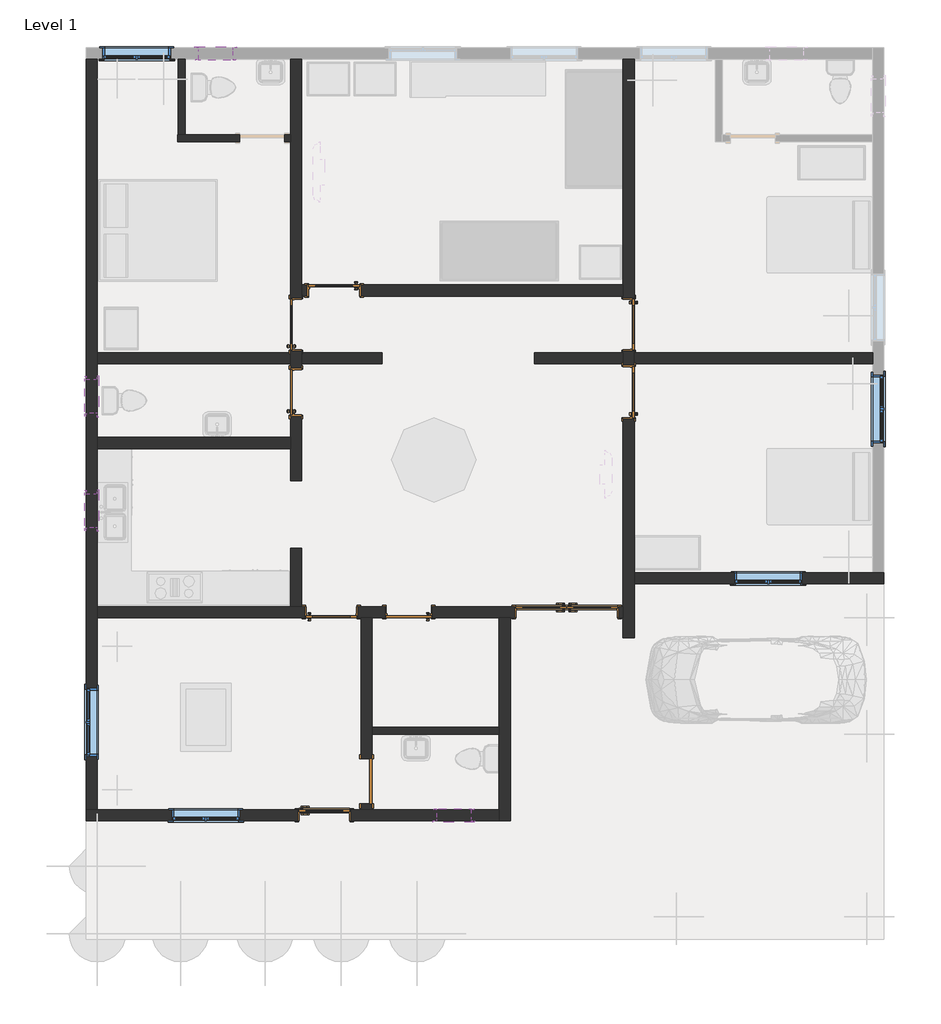
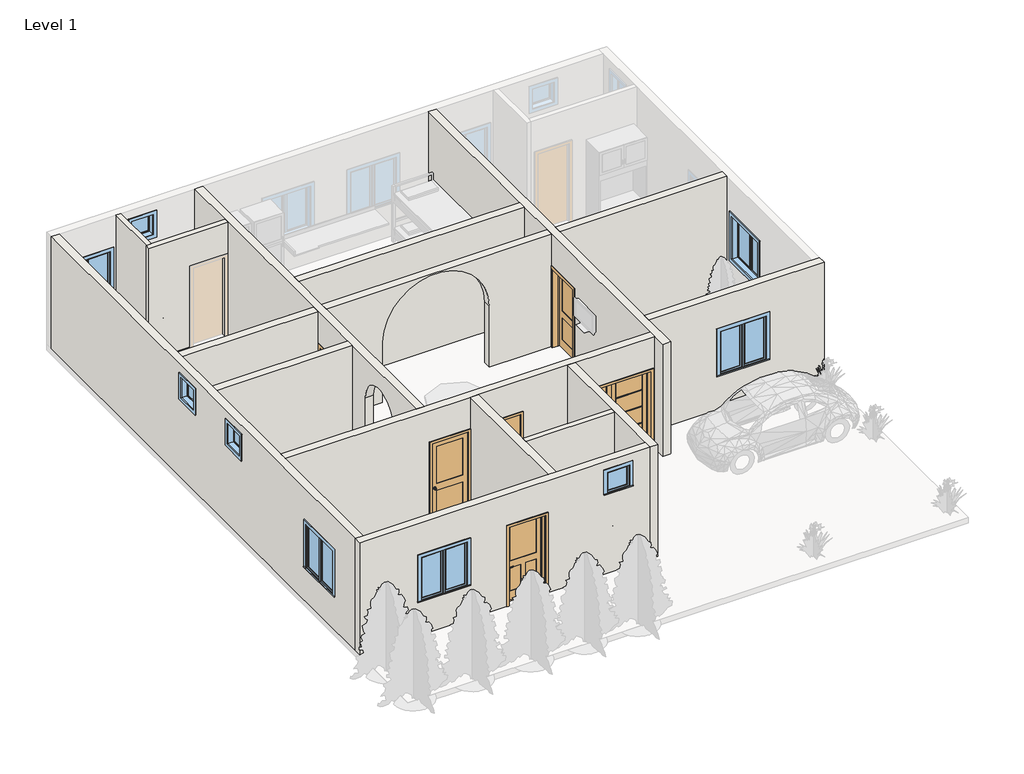
# One storey, part 1 of 2: 14 walls, 10 doors, 9 windows.
"""IFC4 building model written with IfcOpenShell, lengths in millimetres."""

from ifc_helpers import new_model, si_unit, point, frame, frame_2d, origin, origin_with_axes, place, context, project, spatial, polyline, circle_curve, trimmed, segment, composite_curve, outline, extrude, faceted_brep, transform, mapped, element, save
from ifc_brep_helpers import plane_surface, revolved_surface, advanced_brep
from components import door_e879f077, door_06d7e188, door_6f959a6d, door_387d6dd4, door_e4576485, door_70ddef25, window_0862ab64, window_e41d21a6

model = new_model("IFC4")

# Units and contexts
model_context = context("Model", 3, world=origin())
ifc_project = project(units=[si_unit("LENGTHUNIT", "METRE", prefix="MILLI")], contexts=[model_context])

# Site, building, storey
site = spatial("IfcSite", under=ifc_project)
building = spatial("IfcBuilding", under=site)
storey = spatial("IfcBuildingStorey", under=building, Name="Level 1", Elevation=0.0)

# Doors
placement = place(None, origin())
door_shape = door_e879f077(model_context)
element("IfcDoor", 1, ObjectType="36\" x 84\"", at=placement, inside=storey, context=model_context, shape_type="MappedRepresentation", body=[
    mapped(door_shape, transform((1274.4768082, -2194.7262669, 0.0), x_axis=(-1.0, 0.0, 0.0), y_axis=(0.0, -1.0, 0.0), z_axis=(0.0, 0.0, 1.0))),
])
door_2_shape = door_06d7e188(model_context)
element("IfcDoor", 2, ObjectType="Door-Exterior-Double-Full Glass-Wood_Clad : 72\" x 84\"", at=placement, inside=storey, context=model_context, shape_type="MappedRepresentation", body=[
    mapped(door_2_shape, transform((5643.2768082, 1462.8737331, 0.0), x_axis=(1.0, 0.0, 0.0), y_axis=(0.0, 1.0, 0.0), z_axis=(0.0, 0.0, 1.0))),
])
door_3_shape = door_6f959a6d(model_context)
element("IfcDoor", 3, ObjectType="Door-Interior-Single-2_Panel-Wood : 36\" x 84\"", at=placement, inside=storey, context=model_context, shape_type="MappedRepresentation", body=[
    mapped(door_3_shape, transform((6764.0518082, 6641.2987331, 0.0), x_axis=(0.0, -1.0, 0.0), y_axis=(1.0, 0.0, 0.0), z_axis=(0.0, 0.0, 1.0))),
])
element("IfcDoor", 4, ObjectType="Door-Interior-Single-2_Panel-Wood : 36\" x 84\"", at=placement, inside=storey, context=model_context, shape_type="MappedRepresentation", body=[
    mapped(door_3_shape, transform((763.3018082, 6641.2987331, 0.0), x_axis=(0.0, 1.0, 0.0), y_axis=(-1.0, 0.0, 0.0), z_axis=(0.0, 0.0, 1.0))),
])
door_4_shape = door_387d6dd4(model_context)
element("IfcDoor", 5, ObjectType="Door-Interior-Single-2_Panel-Wood : 36\" x 84\"", at=placement, inside=storey, context=model_context, shape_type="MappedRepresentation", body=[
    mapped(door_4_shape, transform((1452.2768082, 7254.0737331, 0.0), x_axis=(-1.0, 0.0, 0.0), y_axis=(0.0, -1.0, 0.0), z_axis=(0.0, 0.0, 1.0))),
])
element("IfcDoor", 6, ObjectType="Door-Interior-Single-2_Panel-Wood : 36\" x 84\"", at=placement, inside=storey, context=model_context, shape_type="MappedRepresentation", body=[
    mapped(door_4_shape, transform((6764.0518082, 5422.0987331, 0.0), x_axis=(0.0, 1.0, 0.0), y_axis=(-1.0, 0.0, 0.0), z_axis=(0.0, 0.0, 1.0))),
])
element("IfcDoor", 7, ObjectType="Door-Interior-Single-2_Panel-Wood : 36\" x 84\"", at=placement, inside=storey, context=model_context, shape_type="MappedRepresentation", body=[
    mapped(door_4_shape, transform((1401.4768082, 1456.5237331, 0.0), x_axis=(1.0, 0.0, 0.0), y_axis=(0.0, 1.0, 0.0), z_axis=(0.0, 0.0, 1.0))),
])
door_5_shape = door_e4576485(model_context)
element("IfcDoor", 8, ObjectType="Door-Interior-Single-Flush_Panel-Wood : 32\" x 84\"", at=placement, inside=storey, context=model_context, shape_type="MappedRepresentation", body=[
    mapped(door_5_shape, transform((763.3018082, 5422.0987331, 0.0), x_axis=(0.0, 1.0, 0.0), y_axis=(-1.0, 0.0, 0.0), z_axis=(0.0, 0.0, 1.0))),
])
element("IfcDoor", 9, ObjectType="Door-Interior-Single-Flush_Panel-Wood : 32\" x 84\"", at=placement, inside=storey, context=model_context, shape_type="MappedRepresentation", body=[
    mapped(door_5_shape, transform((2798.4768082, 1456.5237331, 0.0), x_axis=(-1.0, 0.0, 0.0), y_axis=(0.0, -1.0, 0.0), z_axis=(0.0, 0.0, 1.0))),
])
door_6_shape = door_70ddef25(model_context)
element("IfcDoor", 10, ObjectType="Door-Single-Panel : 32\" x 84\"", at=placement, inside=storey, context=model_context, shape_type="MappedRepresentation", body=[
    mapped(door_6_shape, transform((2036.4768082, -1588.3012669, 0.0), x_axis=(0.0, -1.0, 0.0), y_axis=(1.0, 0.0, 0.0), z_axis=(0.0, 0.0, 1.0))),
])

# Walls
element("IfcWall", 11, ObjectType="Generic - 5\"", at=placement, inside=storey, context=model_context, shape_type="Brep", body=[
    faceted_brep([(563.2768082, 9930.5987331, 2133.6), (563.2768082, 9930.5987331, 0.0), (664.8768082, 9930.5987331, 0.0), (664.8768082, 9930.5987331, 3048.0), (-1367.1231918, 9930.5987331, 3048.0), (-1367.1231918, 9930.5987331, 0.0), (-249.5231918, 9930.5987331, 0.0), (-249.5231918, 9930.5987331, 2133.6), (664.8768082, 10057.5987331, 0.0), (563.2768082, 10057.5987331, 0.0), (563.2768082, 10057.5987331, 2133.6), (-249.5231918, 10057.5987331, 2133.6), (-249.5231918, 10057.5987331, 0.0), (-1227.4231918, 10057.5987331, 0.0), (-1354.4231918, 10057.5987331, 0.0), (-1367.1231918, 10057.5987331, 0.0), (-1367.1231918, 10057.5987331, 3048.0), (-1354.4231918, 10057.5987331, 3048.0), (-1227.4231918, 10057.5987331, 3048.0), (664.8768082, 10057.5987331, 3048.0)], [[[0, 1, 2, 3, 4, 5, 6, 7]], [[8, 9, 10, 11, 12, 13, 14, 15, 16, 17, 18, 19]], [[6, 5, 15, 14, 13, 12]], [[2, 1, 9, 8]], [[4, 3, 19, 18, 17, 16]], [[5, 4, 16, 15]], [[3, 2, 8, 19]], [[10, 9, 1, 0]], [[11, 10, 0, 7]], [[12, 11, 7, 6]]]),
])
element("IfcWall", 12, ObjectType="Generic - 5\"", at=placement, inside=storey, context=model_context, shape_type="SweptSolid", body=[
    extrude(outline(polyline([(-1227.4231918, 11416.4987331), (-1227.4231918, 10057.5987331), (-1354.4231918, 10057.5987331), (-1354.4231918, 11416.4987331), (-1227.4231918, 11416.4987331)])), origin_with_axes(), (0.0, 0.0, 1.0), 3048.0),
])
element("IfcWall", 13, ObjectType="Generic - 5\"", at=placement, inside=storey, context=model_context, shape_type="SweptSolid", body=[
    extrude(outline(polyline([(4424.0768082, -737.4012669), (2138.0768082, -737.4012669), (2138.0768082, -610.4012669), (4424.0768082, -610.4012669), (4424.0768082, -737.4012669)])), origin_with_axes(), (0.0, 0.0, 1.0), 3048.0),
])
element("IfcWall", 14, ObjectType="Generic - 8\"", at=placement, inside=storey, context=model_context, shape_type="Brep", body=[
    faceted_brep([(6659.2768082, 1002.4987331, 0.0), (6659.2768082, 1002.4987331, 3048.0), (6659.2768082, 1358.0987331, 3048.0), (6659.2768082, 1561.2987331, 3048.0), (6659.2768082, 5930.0987331, 3048.0), (6659.2768082, 6133.2987331, 3048.0), (6659.2768082, 7149.2987331, 3048.0), (6659.2768082, 7352.4987331, 3048.0), (6659.2768082, 11416.4987331, 3048.0), (6659.2768082, 11416.4987331, 0.0), (6659.2768082, 7352.4987331, 0.0), (6659.2768082, 7149.2987331, 0.0), (6659.2768082, 7123.8987331, 0.0), (6659.2768082, 7123.8987331, 2159.0), (6659.2768082, 6158.6987331, 2159.0), (6659.2768082, 6158.6987331, 0.0), (6659.2768082, 6133.2987331, 0.0), (6659.2768082, 5930.0987331, 0.0), (6659.2768082, 5904.6987331, 0.0), (6659.2768082, 5904.6987331, 2159.0), (6659.2768082, 4939.4987331, 2159.0), (6659.2768082, 4939.4987331, 0.0), (6659.2768082, 1561.2987331, 0.0), (6659.2768082, 1358.0987331, 0.0), (6862.4768082, 1002.4987331, 3048.0), (6862.4768082, 1002.4987331, 0.0), (6862.4768082, 1967.6987331, 0.0), (6862.4768082, 2170.8987331, 0.0), (6862.4768082, 4939.4987331, 0.0), (6862.4768082, 4939.4987331, 2159.0), (6862.4768082, 5904.6987331, 2159.0), (6862.4768082, 5904.6987331, 0.0), (6862.4768082, 5930.0987331, 0.0), (6862.4768082, 6133.2987331, 0.0), (6862.4768082, 6158.6987331, 0.0), (6862.4768082, 6158.6987331, 2159.0), (6862.4768082, 7123.8987331, 2159.0), (6862.4768082, 7123.8987331, 0.0), (6862.4768082, 11416.4987331, 0.0), (6862.4768082, 11416.4987331, 3048.0), (6862.4768082, 6133.2987331, 3048.0), (6862.4768082, 5930.0987331, 3048.0), (6862.4768082, 2170.8987331, 3048.0), (6862.4768082, 1967.6987331, 3048.0)], [[[0, 1, 2, 3, 4, 5, 6, 7, 8, 9, 10, 11, 12, 13, 14, 15, 16, 17, 18, 19, 20, 21, 22, 23]], [[24, 25, 26, 27, 28, 29, 30, 31, 32, 33, 34, 35, 36, 37, 38, 39, 40, 41, 42, 43]], [[25, 0, 23, 22, 21, 28, 27, 26]], [[9, 38, 37, 12, 11, 10]], [[15, 34, 33, 32, 31, 18, 17, 16]], [[1, 0, 25, 24]], [[8, 7, 6, 5, 4, 3, 2, 1, 24, 43, 42, 41, 40, 39]], [[9, 8, 39, 38]], [[14, 35, 34, 15]], [[35, 14, 13, 36]], [[36, 13, 12, 37]], [[30, 19, 18, 31]], [[19, 30, 29, 20]], [[20, 29, 28, 21]]]),
])
element("IfcWall", 15, ObjectType="Generic - 8\"", at=placement, inside=storey, context=model_context, shape_type="SweptSolid", body=[
    extrude(outline(polyline([(-2814.9231918, 5930.0987331), (-2814.9231918, 6133.2987331), (664.8768082, 6133.2987331), (664.8768082, 5930.0987331), (-2814.9231918, 5930.0987331)])), origin_with_axes(), (0.0, 0.0, 1.0), 3048.0),
    extrude(outline(polyline([(11155.0768082, 6133.2987331), (11155.0768082, 5930.0987331), (6862.4768082, 5930.0987331), (6862.4768082, 6133.2987331), (11155.0768082, 6133.2987331)])), origin_with_axes(), (0.0, 0.0, 1.0), 3048.0),
    extrude(outline(composite_curve([segment(polyline([(0.0, 6659.2768082), (3048.0, 6659.2768082), (3048.0, 868.0768082), (0.0, 868.0768082), (0.0, 2315.8768082), (1646.356949, 2315.8768082)]), True, "CONTINUOUS"), segment(trimmed(circle_curve(frame_2d((1646.356949, 3687.4768082)), 1371.6), [point((1646.356949, 2315.8768082))], [point((1646.356949, 5059.0768082))], True, "CARTESIAN"), True, "CONTINUOUS"), segment(polyline([(1646.356949, 5059.0768082), (0.0, 5059.0768082), (0.0, 6659.2768082)]), True, "CONTINUOUS")], self_intersect=False)), frame((0.0, 5930.0987331, 0.0), z_axis=(0.0, 1.0, 0.0), x_axis=(0.0, 0.0, 1.0)), (0.0, 0.0, 1.0), 203.2),
])
element("IfcWall", 16, ObjectType="Generic - 8\"", at=placement, inside=storey, context=model_context, shape_type="Brep", body=[
    faceted_brep([(6659.2768082, 1358.0987331, 3048.0), (4627.2768082, 1358.0987331, 3048.0), (4424.0768082, 1358.0987331, 3048.0), (2138.0768082, 1358.0987331, 3048.0), (1934.8768082, 1358.0987331, 3048.0), (-2814.9231918, 1358.0987331, 3048.0), (-2814.9231918, 1358.0987331, 0.0), (918.8768082, 1358.0987331, 0.0), (918.8768082, 1358.0987331, 2159.0), (1884.0768082, 1358.0987331, 2159.0), (1884.0768082, 1358.0987331, 0.0), (1934.8768082, 1358.0987331, 0.0), (2138.0768082, 1358.0987331, 0.0), (2366.6768082, 1358.0987331, 0.0), (2366.6768082, 1358.0987331, 2159.0), (3230.2768082, 1358.0987331, 2159.0), (3230.2768082, 1358.0987331, 0.0), (4424.0768082, 1358.0987331, 0.0), (4627.2768082, 1358.0987331, 0.0), (4703.4768082, 1358.0987331, 0.0), (4703.4768082, 1358.0987331, 2159.0), (6583.0768082, 1358.0987331, 2159.0), (6583.0768082, 1358.0987331, 0.0), (6659.2768082, 1358.0987331, 0.0), (-2814.9231918, 1561.2987331, 3048.0), (664.8768082, 1561.2987331, 3048.0), (868.0768082, 1561.2987331, 3048.0), (6659.2768082, 1561.2987331, 3048.0), (6659.2768082, 1561.2987331, 0.0), (6583.0768082, 1561.2987331, 0.0), (6583.0768082, 1561.2987331, 2159.0), (4703.4768082, 1561.2987331, 2159.0), (4703.4768082, 1561.2987331, 0.0), (3230.2768082, 1561.2987331, 0.0), (3230.2768082, 1561.2987331, 2159.0), (2366.6768082, 1561.2987331, 2159.0), (2366.6768082, 1561.2987331, 0.0), (1884.0768082, 1561.2987331, 0.0), (1884.0768082, 1561.2987331, 2159.0), (918.8768082, 1561.2987331, 2159.0), (918.8768082, 1561.2987331, 0.0), (868.0768082, 1561.2987331, 0.0), (664.8768082, 1561.2987331, 0.0), (-2814.9231918, 1561.2987331, 0.0)], [[[0, 1, 2, 3, 4, 5, 6, 7, 8, 9, 10, 11, 12, 13, 14, 15, 16, 17, 18, 19, 20, 21, 22, 23]], [[24, 25, 26, 27, 28, 29, 30, 31, 32, 33, 34, 35, 36, 37, 38, 39, 40, 41, 42, 43]], [[6, 43, 42, 41, 40, 7]], [[28, 23, 22, 29]], [[10, 37, 36, 13, 12, 11]], [[32, 19, 18, 17, 16, 33]], [[5, 4, 3, 2, 1, 0, 27, 26, 25, 24]], [[6, 5, 24, 43]], [[0, 23, 28, 27]], [[10, 9, 38, 37]], [[9, 8, 39, 38]], [[8, 7, 40, 39]], [[21, 30, 29, 22]], [[30, 21, 20, 31]], [[31, 20, 19, 32]], [[35, 14, 13, 36]], [[14, 35, 34, 15]], [[15, 34, 33, 16]]]),
])
element("IfcWall", 17, ObjectType="Generic - 8\"", at=placement, inside=storey, context=model_context, shape_type="Brep", body=[
    faceted_brep([(6862.4768082, 1967.6987331, 0.0), (11358.2768082, 1967.6987331, 0.0), (11358.2768082, 1967.6987331, 3048.0), (6862.4768082, 1967.6987331, 3048.0), (8665.8768082, 1967.6987331, 2133.6), (9885.0768082, 1967.6987331, 2133.6), (9885.0768082, 1967.6987331, 914.4), (8665.8768082, 1967.6987331, 914.4), (6862.4768082, 2170.8987331, 0.0), (6862.4768082, 2170.8987331, 3048.0), (11155.0768082, 2170.8987331, 3048.0), (11358.2768082, 2170.8987331, 3048.0), (11358.2768082, 2170.8987331, 0.0), (11155.0768082, 2170.8987331, 0.0), (8665.8768082, 2170.8987331, 2133.6), (8665.8768082, 2170.8987331, 914.4), (9885.0768082, 2170.8987331, 914.4), (9885.0768082, 2170.8987331, 2133.6)], [[[0, 1, 2, 3], [4, 5, 6, 7]], [[8, 9, 10, 11, 12, 13], [14, 15, 16, 17]], [[1, 0, 8, 13, 12]], [[3, 2, 11, 10, 9]], [[0, 3, 9, 8]], [[2, 1, 12, 11]], [[15, 14, 4, 7]], [[16, 15, 7, 6]], [[17, 16, 6, 5]], [[14, 17, 5, 4]]]),
])
element("IfcWall", 18, ObjectType="Generic - 8\"", at=placement, inside=storey, context=model_context, shape_type="SweptSolid", body=[
    extrude(outline(polyline([(3048.0, 6659.2768082), (3048.0, 868.0768082), (0.0, 868.0768082), (0.0, 969.6768082), (2159.0, 969.6768082), (2159.0, 1934.8768082), (0.0, 1934.8768082), (0.0, 6659.2768082), (3048.0, 6659.2768082)])), frame((0.0, 7149.2987331, 0.0), z_axis=(0.0, 1.0, 0.0), x_axis=(0.0, 0.0, 1.0)), (0.0, 0.0, 1.0), 203.2),
])
element("IfcWall", 19, ObjectType="Generic - 8\"", at=placement, inside=storey, context=model_context, shape_type="SweptSolid", body=[
    extrude(outline(polyline([(664.8768082, 4406.0987331), (-2814.9231918, 4406.0987331), (-2814.9231918, 4609.2987331), (664.8768082, 4609.2987331), (664.8768082, 4406.0987331)])), origin_with_axes(), (0.0, 0.0, 1.0), 3048.0),
])
element("IfcWall", 20, ObjectType="Generic - 8\"", at=placement, inside=storey, context=model_context, shape_type="Brep", body=[
    faceted_brep([(4424.0768082, -2299.5012669, 3048.0), (-3018.1231918, -2299.5012669, 3048.0), (-3018.1231918, -2299.5012669, 0.0), (791.8768082, -2299.5012669, 0.0), (791.8768082, -2299.5012669, 2159.0), (1757.0768082, -2299.5012669, 2159.0), (1757.0768082, -2299.5012669, 0.0), (4424.0768082, -2299.5012669, 0.0), (-1468.7231918, -2299.5012669, 2133.6), (-249.5231918, -2299.5012669, 2133.6), (-249.5231918, -2299.5012669, 914.4), (-1468.7231918, -2299.5012669, 914.4), (3306.4768082, -2299.5012669, 2768.6), (3916.0768082, -2299.5012669, 2768.6), (3916.0768082, -2299.5012669, 2159.0), (3306.4768082, -2299.5012669, 2159.0), (-3018.1231918, -2096.3012669, 3048.0), (-2814.9231918, -2096.3012669, 3048.0), (1934.8768082, -2096.3012669, 3048.0), (2138.0768082, -2096.3012669, 3048.0), (4424.0768082, -2096.3012669, 3048.0), (4424.0768082, -2096.3012669, 0.0), (2138.0768082, -2096.3012669, 0.0), (1934.8768082, -2096.3012669, 0.0), (1757.0768082, -2096.3012669, 0.0), (1757.0768082, -2096.3012669, 2159.0), (791.8768082, -2096.3012669, 2159.0), (791.8768082, -2096.3012669, 0.0), (-2814.9231918, -2096.3012669, 0.0), (-3018.1231918, -2096.3012669, 0.0), (-1468.7231918, -2096.3012669, 2133.6), (-1468.7231918, -2096.3012669, 914.4), (-249.5231918, -2096.3012669, 914.4), (-249.5231918, -2096.3012669, 2133.6), (3306.4768082, -2096.3012669, 2768.6), (3306.4768082, -2096.3012669, 2159.0), (3916.0768082, -2096.3012669, 2159.0), (3916.0768082, -2096.3012669, 2768.6)], [[[0, 1, 2, 3, 4, 5, 6, 7], [8, 9, 10, 11], [12, 13, 14, 15]], [[16, 17, 18, 19, 20, 21, 22, 23, 24, 25, 26, 27, 28, 29], [30, 31, 32, 33], [34, 35, 36, 37]], [[21, 7, 6, 24, 23, 22]], [[2, 29, 28, 27, 3]], [[1, 0, 20, 19, 18, 17, 16]], [[0, 7, 21, 20]], [[2, 1, 16, 29]], [[31, 30, 8, 11]], [[32, 31, 11, 10]], [[33, 32, 10, 9]], [[30, 33, 9, 8]], [[35, 34, 12, 15]], [[36, 35, 15, 14]], [[37, 36, 14, 13]], [[34, 37, 13, 12]], [[26, 4, 3, 27]], [[4, 26, 25, 5]], [[5, 25, 24, 6]]]),
])
element("IfcWall", 21, ObjectType="Generic - 8\"", at=placement, inside=storey, context=model_context, shape_type="AdvancedBrep", body=[
    advanced_brep(
    [(868.0768082, 1561.2987331, 0.0), (868.0768082, 2608.3353114, 0.0), (868.0768082, 2608.3353114, 1981.2), (868.0768082, 3827.5353114, 1981.2), (868.0768082, 3827.5353114, 0.0), (868.0768082, 4990.2987331, 0.0), (868.0768082, 4990.2987331, 2159.0), (868.0768082, 5853.8987331, 2159.0), (868.0768082, 5853.8987331, 0.0), (868.0768082, 5930.0987331, 0.0), (868.0768082, 6133.2987331, 0.0), (868.0768082, 6158.6987331, 0.0), (868.0768082, 6158.6987331, 2159.0), (868.0768082, 7123.8987331, 2159.0), (868.0768082, 7123.8987331, 0.0), (868.0768082, 7149.2987331, 0.0), (868.0768082, 7352.4987331, 0.0), (868.0768082, 11416.4987331, 0.0), (868.0768082, 11416.4987331, 3048.0), (868.0768082, 7352.4987331, 3048.0), (868.0768082, 7149.2987331, 3048.0), (868.0768082, 6133.2987331, 3048.0), (868.0768082, 5930.0987331, 3048.0), (868.0768082, 1561.2987331, 3048.0), (664.8768082, 2608.3353114, 0.0), (664.8768082, 1561.2987331, 0.0), (664.8768082, 1561.2987331, 3048.0), (664.8768082, 4406.0987331, 3048.0), (664.8768082, 4609.2987331, 3048.0), (664.8768082, 5930.0987331, 3048.0), (664.8768082, 6133.2987331, 3048.0), (664.8768082, 9930.5987331, 3048.0), (664.8768082, 10057.5987331, 3048.0), (664.8768082, 11416.4987331, 3048.0), (664.8768082, 11416.4987331, 0.0), (664.8768082, 10057.5987331, 0.0), (664.8768082, 9930.5987331, 0.0), (664.8768082, 7123.8987331, 0.0), (664.8768082, 7123.8987331, 2159.0), (664.8768082, 6158.6987331, 2159.0), (664.8768082, 6158.6987331, 0.0), (664.8768082, 6133.2987331, 0.0), (664.8768082, 5930.0987331, 0.0), (664.8768082, 5853.8987331, 0.0), (664.8768082, 5853.8987331, 2159.0), (664.8768082, 4990.2987331, 2159.0), (664.8768082, 4990.2987331, 0.0), (664.8768082, 4609.2987331, 0.0), (664.8768082, 4406.0987331, 0.0), (664.8768082, 3827.5353114, 0.0), (664.8768082, 3827.5353114, 1981.2), (664.8768082, 2608.3353114, 1981.2)],
    [
        (0, 1),
        (1, 2),
        (2, 3, circle_curve(frame((868.0768082, 3217.9353114, 1981.2), z_axis=(-1.0, 0.0, 0.0), x_axis=(0.0, -1.0, 0.0)), 609.6)),
        (3, 4),
        (4, 5),
        (5, 6),
        (6, 7),
        (7, 8),
        (8, 9),
        (9, 10),
        (10, 11),
        (11, 12),
        (12, 13),
        (13, 14),
        (14, 15),
        (15, 16),
        (16, 17),
        (17, 18),
        (18, 19),
        (19, 20),
        (20, 21),
        (21, 22),
        (22, 23),
        (23, 0),
        (24, 25),
        (25, 26),
        (26, 27),
        (27, 28),
        (28, 29),
        (29, 30),
        (30, 31),
        (31, 32),
        (32, 33),
        (33, 34),
        (34, 35),
        (35, 36),
        (36, 37),
        (37, 38),
        (38, 39),
        (39, 40),
        (40, 41),
        (41, 42),
        (42, 43),
        (43, 44),
        (44, 45),
        (45, 46),
        (46, 47),
        (47, 48),
        (48, 49),
        (49, 50),
        (50, 51, circle_curve(frame((664.8768082, 3217.9353114, 1981.2), z_axis=(1.0, 0.0, 0.0), x_axis=(0.0, -1.0, 0.0)), 609.6)),
        (51, 24),
        (17, 34),
        (33, 18),
        (23, 26),
        (25, 0),
        (13, 38),
        (37, 14),
        (12, 39),
        (11, 40),
        (24, 1),
        (51, 2),
        (50, 3),
        (49, 4),
        (46, 5),
        (8, 43),
        (7, 44),
        (6, 45),
    ],
    [
        plane_surface(frame((868.0768082, 15886.8987331, 0.0), z_axis=(1.0, 0.0, 0.0), x_axis=(0.0, 1.0, 0.0))),
        plane_surface(frame((664.8768082, 15886.8987331, 0.0), z_axis=(-1.0, 0.0, 0.0), x_axis=(0.0, -1.0, 0.0))),
        plane_surface(frame((-11908.1231918, 11416.4987331, 0.0), z_axis=(0.0, 1.0, 0.0), x_axis=(1.0, 0.0, 0.0))),
        plane_surface(frame((-11908.1231918, 1561.2987331, 0.0), z_axis=(0.0, -1.0, 0.0), x_axis=(-1.0, 0.0, 0.0))),
        plane_surface(frame((2392.0768082, 7123.8987331, 0.0), z_axis=(0.0, -1.0, 0.0), x_axis=(-1.0, 0.0, 0.0))),
        plane_surface(frame((2392.0768082, 7123.8987331, 2159.0), z_axis=(0.0, 0.0, -1.0), x_axis=(-1.0, 0.0, 0.0))),
        plane_surface(frame((2392.0768082, 6158.6987331, 2159.0), z_axis=(0.0, 1.0, 0.0), x_axis=(-1.0, 0.0, 0.0))),
        plane_surface(frame((868.0768082, 1459.6987331, 0.0), z_axis=(0.0, 0.0, -1.0), x_axis=(-1.0, 0.0, 0.0))),
        plane_surface(frame((868.0768082, 11518.0987331, 3048.0), z_axis=(0.0, 0.0, 1.0), x_axis=(-1.0, 0.0, 0.0))),
        plane_surface(frame((868.0768082, 2608.3353114, 0.0), z_axis=(0.0, 1.0, 0.0), x_axis=(-1.0, 0.0, 0.0))),
        revolved_surface(polyline([(664.8768082, 2608.3353114, 1981.2), (868.0768082, 2608.3353114, 1981.2)]), (664.8768082, 3217.9353114, 1981.2), (-1.0, 0.0, 0.0)),
        plane_surface(frame((868.0768082, 3827.5353114, 1981.2), z_axis=(0.0, -1.0, 0.0), x_axis=(-1.0, 0.0, 0.0))),
        plane_surface(frame((868.0768082, 3827.5353114, 0.0), z_axis=(0.0, 0.0, -1.0), x_axis=(-1.0, 0.0, 0.0))),
        plane_surface(frame((2392.0768082, 5853.8987331, 0.0), z_axis=(0.0, -1.0, 0.0), x_axis=(-1.0, 0.0, 0.0))),
        plane_surface(frame((2392.0768082, 5853.8987331, 2159.0), z_axis=(0.0, 0.0, -1.0), x_axis=(-1.0, 0.0, 0.0))),
        plane_surface(frame((2392.0768082, 4990.2987331, 2159.0), z_axis=(0.0, 1.0, 0.0), x_axis=(-1.0, 0.0, 0.0))),
    ],
    [
        (0, [[1, 2, 3, 4, 5, 6, 7, 8, 9, 10, 11, 12, 13, 14, 15, 16, 17, 18, 19, 20, 21, 22, 23, 24]]),
        (1, [[25, 26, 27, 28, 29, 30, 31, 32, 33, 34, 35, 36, 37, 38, 39, 40, 41, 42, 43, 44, 45, 46, 47, 48, 49, 50, 51, 52]]),
        (2, [[-18, 53, -34, 54]]),
        (3, [[-24, 55, -26, 56]]),
        (4, [[57, -38, 58, -14]]),
        (5, [[-57, -13, 59, -39]]),
        (6, [[-59, -12, 60, -40]]),
        (7, [[-1, -56, -25, 61]]),
        (8, [[-23, -22, -21, -20, -19, -54, -33, -32, -31, -30, -29, -28, -27, -55]]),
        (9, [[-2, -61, -52, 62]]),
        (10, [[-3, -62, -51, 63]]),
        (11, [[-4, -63, -50, 64]]),
        (12, [[-64, -49, -48, -47, 65, -5]]),
        (12, [[-60, -11, -10, -9, 66, -43, -42, -41]]),
        (12, [[-53, -17, -16, -15, -58, -37, -36, -35]]),
        (13, [[67, -44, -66, -8]]),
        (14, [[-67, -7, 68, -45]]),
        (15, [[-68, -6, -65, -46]]),
    ],
),
])
element("IfcWall", 22, ObjectType="Generic - 8\"", at=placement, inside=storey, context=model_context, shape_type="Brep", body=[
    faceted_brep([(4424.0768082, 1358.0987331, 0.0), (4424.0768082, -610.4012669, 0.0), (4424.0768082, -737.4012669, 0.0), (4424.0768082, -2096.3012669, 0.0), (4424.0768082, -2299.5012669, 0.0), (4424.0768082, -2299.5012669, 3048.0), (4424.0768082, -2096.3012669, 3048.0), (4424.0768082, -737.4012669, 3048.0), (4424.0768082, -610.4012669, 3048.0), (4424.0768082, 1358.0987331, 3048.0), (4627.2768082, 1358.0987331, 0.0), (4627.2768082, 1358.0987331, 3048.0), (4627.2768082, -2299.5012669, 3048.0), (4627.2768082, -2299.5012669, 0.0)], [[[0, 1, 2, 3, 4, 5, 6, 7, 8, 9]], [[10, 11, 12, 13]], [[4, 3, 2, 1, 0, 10, 13]], [[9, 8, 7, 6, 5, 12, 11]], [[0, 9, 11, 10]], [[5, 4, 13, 12]]]),
])
element("IfcWall", 23, ObjectType="Generic - 8\"", at=placement, inside=storey, context=model_context, shape_type="Brep", body=[
    faceted_brep([(1934.8768082, -1994.7012669, 2133.6), (1934.8768082, -1994.7012669, 0.0), (1934.8768082, -2096.3012669, 0.0), (1934.8768082, -2096.3012669, 3048.0), (1934.8768082, 1358.0987331, 3048.0), (1934.8768082, 1358.0987331, 0.0), (1934.8768082, -1181.9012669, 0.0), (1934.8768082, -1181.9012669, 2133.6), (2138.0768082, -2096.3012669, 0.0), (2138.0768082, -1994.7012669, 0.0), (2138.0768082, -1994.7012669, 2133.6), (2138.0768082, -1181.9012669, 2133.6), (2138.0768082, -1181.9012669, 0.0), (2138.0768082, -737.4012669, 0.0), (2138.0768082, -610.4012669, 0.0), (2138.0768082, 1358.0987331, 0.0), (2138.0768082, 1358.0987331, 3048.0), (2138.0768082, -610.4012669, 3048.0), (2138.0768082, -737.4012669, 3048.0), (2138.0768082, -2096.3012669, 3048.0)], [[[0, 1, 2, 3, 4, 5, 6, 7]], [[8, 9, 10, 11, 12, 13, 14, 15, 16, 17, 18, 19]], [[6, 5, 15, 14, 13, 12]], [[2, 1, 9, 8]], [[4, 3, 19, 18, 17, 16]], [[5, 4, 16, 15]], [[3, 2, 8, 19]], [[10, 9, 1, 0]], [[11, 10, 0, 7]], [[12, 11, 7, 6]]]),
])
element("IfcWall", 24, ObjectType="Generic - 8\" - Filled", at=placement, inside=storey, context=model_context, shape_type="Brep", body=[
    faceted_brep([(-2814.9231918, -2096.3012669, 0.0), (-2814.9231918, 1358.0987331, 0.0), (-2814.9231918, 1561.2987331, 0.0), (-2814.9231918, 4406.0987331, 0.0), (-2814.9231918, 4609.2987331, 0.0), (-2814.9231918, 5930.0987331, 0.0), (-2814.9231918, 6133.2987331, 0.0), (-2814.9231918, 11416.4987331, 0.0), (-2814.9231918, 11416.4987331, 3048.0), (-2814.9231918, 6133.2987331, 3048.0), (-2814.9231918, 5930.0987331, 3048.0), (-2814.9231918, 4609.2987331, 3048.0), (-2814.9231918, 4406.0987331, 3048.0), (-2814.9231918, 1561.2987331, 3048.0), (-2814.9231918, 1358.0987331, 3048.0), (-2814.9231918, -2096.3012669, 3048.0), (-2814.9231918, 88.0987331, 2133.6), (-2814.9231918, 88.0987331, 914.4), (-2814.9231918, -1131.1012669, 914.4), (-2814.9231918, -1131.1012669, 2133.6), (-2814.9231918, 2983.6987331, 2768.6), (-2814.9231918, 3593.2987331, 2768.6), (-2814.9231918, 3593.2987331, 2159.0), (-2814.9231918, 2983.6987331, 2159.0), (-2814.9231918, 5041.0987331, 2768.6), (-2814.9231918, 5650.6987331, 2768.6), (-2814.9231918, 5650.6987331, 2159.0), (-2814.9231918, 5041.0987331, 2159.0), (-3018.1231918, -2096.3012669, 0.0), (-3018.1231918, -2096.3012669, 3048.0), (-3018.1231918, 11416.4987331, 3048.0), (-3018.1231918, 11416.4987331, 0.0), (-3018.1231918, 88.0987331, 2133.6), (-3018.1231918, -1131.1012669, 2133.6), (-3018.1231918, -1131.1012669, 914.4), (-3018.1231918, 88.0987331, 914.4), (-3018.1231918, 2983.6987331, 2768.6), (-3018.1231918, 2983.6987331, 2159.0), (-3018.1231918, 3593.2987331, 2159.0), (-3018.1231918, 3593.2987331, 2768.6), (-3018.1231918, 5041.0987331, 2768.6), (-3018.1231918, 5041.0987331, 2159.0), (-3018.1231918, 5650.6987331, 2159.0), (-3018.1231918, 5650.6987331, 2768.6)], [[[0, 1, 2, 3, 4, 5, 6, 7, 8, 9, 10, 11, 12, 13, 14, 15], [16, 17, 18, 19], [20, 21, 22, 23], [24, 25, 26, 27]], [[28, 29, 30, 31], [32, 33, 34, 35], [36, 37, 38, 39], [40, 41, 42, 43]], [[7, 6, 5, 4, 3, 2, 1, 0, 28, 31]], [[15, 14, 13, 12, 11, 10, 9, 8, 30, 29]], [[8, 7, 31, 30]], [[0, 15, 29, 28]], [[17, 16, 32, 35]], [[18, 17, 35, 34]], [[19, 18, 34, 33]], [[16, 19, 33, 32]], [[37, 36, 20, 23]], [[38, 37, 23, 22]], [[39, 38, 22, 21]], [[36, 39, 21, 20]], [[41, 40, 24, 27]], [[42, 41, 27, 26]], [[43, 42, 26, 25]], [[40, 43, 25, 24]]]),
])

# Windows
window_shape = window_0862ab64(model_context)
element("IfcWindow", 25, ObjectType="Casement Dbl with Trim : 48\" x 48\"", at=placement, inside=storey, context=model_context, shape_type="MappedRepresentation", body=[
    mapped(window_shape, transform((-2103.7231918, 11537.1487331, 0.0), x_axis=(-1.0, 0.0, 0.0), y_axis=(0.0, -1.0, 0.0), z_axis=(0.0, 0.0, 1.0))),
])
element("IfcWindow", 26, ObjectType="Casement Dbl with Trim : 48\" x 48\"", at=placement, inside=storey, context=model_context, shape_type="MappedRepresentation", body=[
    mapped(window_shape, transform((11237.6268082, 5117.2987331, 0.0), x_axis=(0.0, -1.0, 0.0), y_axis=(1.0, 0.0, 0.0), z_axis=(0.0, 0.0, 1.0))),
])
element("IfcWindow", 27, ObjectType="Casement Dbl with Trim : 48\" x 48\"", at=placement, inside=storey, context=model_context, shape_type="MappedRepresentation", body=[
    mapped(window_shape, transform((9275.4768082, 2088.3487331, 0.0), x_axis=(-1.0, 0.0, 0.0), y_axis=(0.0, -1.0, 0.0), z_axis=(0.0, 0.0, 1.0))),
])
element("IfcWindow", 28, ObjectType="Casement Dbl with Trim : 48\" x 48\"", at=placement, inside=storey, context=model_context, shape_type="MappedRepresentation", body=[
    mapped(window_shape, transform((-859.1231918, -2178.8512669, 0.0), x_axis=(-1.0, 0.0, 0.0), y_axis=(0.0, -1.0, 0.0), z_axis=(0.0, 0.0, 1.0))),
])
element("IfcWindow", 29, ObjectType="Casement Dbl with Trim : 48\" x 48\"", at=placement, inside=storey, context=model_context, shape_type="MappedRepresentation", body=[
    mapped(window_shape, transform((-2897.4731918, -521.5012669, 0.0), x_axis=(0.0, 1.0, 0.0), y_axis=(-1.0, 0.0, 0.0), z_axis=(0.0, 0.0, 1.0))),
])
window_2_shape = window_e41d21a6(model_context)
element("IfcWindow", 30, ObjectType="Transom with Trim : 24\" x 24\"", at=placement, inside=storey, context=model_context, shape_type="MappedRepresentation", body=[
    mapped(window_2_shape, transform((-643.2231918, 11518.0987331, 0.0), x_axis=(1.0, 0.0, 0.0), y_axis=(0.0, 1.0, 0.0), z_axis=(0.0, 0.0, 1.0))),
])
element("IfcWindow", 31, ObjectType="Transom with Trim : 24\" x 24\"", at=placement, inside=storey, context=model_context, shape_type="MappedRepresentation", body=[
    mapped(window_2_shape, transform((3573.1768082, -2197.9012669, 0.0), x_axis=(-1.0, 0.0, 0.0), y_axis=(0.0, -1.0, 0.0), z_axis=(0.0, 0.0, 1.0))),
])
element("IfcWindow", 32, ObjectType="Transom with Trim : 24\" x 24\"", at=placement, inside=storey, context=model_context, shape_type="MappedRepresentation", body=[
    mapped(window_2_shape, transform((-2916.5231918, 3250.3987331, 0.0), x_axis=(0.0, -1.0, 0.0), y_axis=(1.0, 0.0, 0.0), z_axis=(0.0, 0.0, 1.0))),
])
element("IfcWindow", 33, ObjectType="Transom with Trim : 24\" x 24\"", at=placement, inside=storey, context=model_context, shape_type="MappedRepresentation", body=[
    mapped(window_2_shape, transform((-2916.5231918, 5307.7987331, 0.0), x_axis=(0.0, -1.0, 0.0), y_axis=(1.0, 0.0, 0.0), z_axis=(0.0, 0.0, 1.0))),
])

save(model, "model.ifc")

# Revit data of these elements
# Type "36\" x 84\""
#   Type Mark = "15"
#   Assembly Code = "B2030100"
#   Analytic Construction = "French door, wood frame with single glass"
#   Top Rail = 0' - 4 3/4"
#   Threshold Offset [instance default] = 0' - 0 1/2"
#   Thickness = 0' - 1 3/8"
#   Thermal Resistance (R) = 1.0696 (h·ft²·°F)/BTU
#   Swing Angle [instance default] = 90.00°
#   Stiles = 0' - 4 3/4"
#   Rough Width = 3' - 2"
#   Rough Height = 7' - 1"
#   Lock Rail = 0' - 7 1/8"
#   Height = 7' - 0"
#   Width = 3' - 0"
#   Heat Transfer Coefficient (U) = 0.9350 BTU/(h·ft²·°F)
#   Door Offset [instance default] = 0' - 0"
#   Bottom Rail = 0' - 9 1/2"
#   Threshold [instance default] = yes
#   Function = 1
#   Exterior Trim [instance default] = yes
#   Trim Material = Cherry
#   Threshold Material = Cherry
#   Panel Material = Cherry
#   Glazing = Glass
#   Frame Material = Cherry
#   Door Handle Material = Aluminum
#   Visual Light Transmittance = 0
#   Solar Heat Gain Coefficient = 0
#   Wall Closure = (empty or 0)
#   Construction Type = (empty or 0)
# Type "Door-Exterior-Double-Full Glass-Wood_Clad : 72\" x 84\""
#   Type Mark = "8"
#   Assembly Code = "B2030100"
#   Analytic Construction = "French door, wood frame with double glass"
#   Top Rail = 0' - 4 11/16"
#   Threshold Offset [instance default] = 0' - 0 1/2"
#   Thickness = 0' - 1 3/8"
#   Thermal Resistance (R) = 1.9158 (h·ft²·°F)/BTU
#   Swing Angle [instance default] = 90.00°
#   Stiles = 0' - 4 3/4"
#   Rough Width = 6' - 2"
#   Rough Height = 7' - 1"
#   Panel Width = 3' - 0"
#   Door Offset [instance default] = 0' - 0"
#   Height = 7' - 0"
#   Width = 6' - 0"
#   Heat Transfer Coefficient (U) = 0.5220 BTU/(h·ft²·°F)
#   Bottom Rail = 0' - 9 1/8"
#   Exterior Trim [instance default] = yes
#   Threshold [instance default] = yes
#   Show Grill [instance default] = yes
#   Function = 1
#   Trim Material = Cherry
#   Threshold Material = Cherry
#   Panel Material = Cherry
#   Glazing = Glass
#   Frame Material = Cherry
#   Door Handle Material = Aluminum
#   Visual Light Transmittance = 0
#   Solar Heat Gain Coefficient = 0
#   Wall Closure = (empty or 0)
#   Construction Type = (empty or 0)
# Type "Door-Interior-Single-2_Panel-Wood : 36\" x 84\""
#   Type Mark = "9"
#   Assembly Code = "C1020300"
#   Analytic Construction = "Wooden"
#   Top Rail = 0' - 4 11/16"
#   Thickness = 0' - 1 3/8"
#   Thermal Resistance (R) = 2.5876 (h·ft²·°F)/BTU
#   Swing Angle [instance default] = 90.00°
#   Stiles = 0' - 4 3/4"
#   Rough Width = 3' - 2"
#   Rough Height = 7' - 1"
#   Lock Rail = 0' - 7 1/2"
#   Height = 7' - 0"
#   Width = 3' - 0"
#   Heat Transfer Coefficient (U) = 0.3865 BTU/(h·ft²·°F)
#   Bottom Rail = 0' - 9 1/8"
#   Trim Material = Cherry
#   Panel Material = Cherry
#   Frame Material = Cherry
#   Door Handle Material = Aluminum
#   Visual Light Transmittance = 0
#   Solar Heat Gain Coefficient = 0
#   Wall Closure = (empty or 0)
#   Function = (empty or 0)
# Type "Door-Interior-Single-Flush_Panel-Wood : 32\" x 84\""
#   Type Mark = "13"
#   Assembly Code = "C1020300"
#   Analytic Construction = "Wooden"
#   Thickness = 0' - 1 3/8"
#   Thermal Resistance (R) = 2.5876 (h·ft²·°F)/BTU
#   Swing Angle [instance default] = 90.00°
#   Rough Width = 2' - 10"
#   Rough Height = 7' - 1"
#   Height = 7' - 0"
#   Width = 2' - 8"
#   Heat Transfer Coefficient (U) = 0.3865 BTU/(h·ft²·°F)
#   Trim Material = Cherry
#   Panel Material = Cherry
#   Frame Material = Cherry
#   Door Handle Material = Aluminum
#   Visual Light Transmittance = 0
#   Solar Heat Gain Coefficient = 0
#   Wall Closure = (empty or 0)
#   Function = (empty or 0)
# Type "Door-Single-Panel : 32\" x 84\""
#   Type Mark = "11"
#   Construction Type Id = "DOOR"
#   Assembly Code = "C1020300"
#   Analytic Construction = "Wooden"
#   Thickness = 0' - 2"
#   Thermal Resistance (R) = 2.5876 (h·ft²·°F)/BTU
#   Swing Angle [instance default] = 90.00°
#   Heat Transfer Coefficient (U) = 0.3865 BTU/(h·ft²·°F)
#   Height = 7' - 0"
#   Trim Projection Ext = 0' - 1"
#   Trim Projection Int = 0' - 1"
#   Trim Width = 0' - 3"
#   Width = 2' - 8"
#   Define Thermal Properties by = 1
#   Panel Material = Wood - Birch - Solid Stained Light Low Gloss
#   Trim Material = Paint - Sienna
#   Visual Light Transmittance = 0
#   Solar Heat Gain Coefficient = 0
#   Function = (empty or 0)
#   Wall Closure = (empty or 0)
# Type "Generic - 5\""
#   Assembly Code = "B2010"
#   Layers, outside or top first: 0' - 5" no material (function 1)
# Type "Generic - 8\""
#   Assembly Code = "B2010"
#   Layers, outside or top first: 0' - 8" "Paint - Sienna" (function 1)
# Type "Generic - 8\" - Filled"
#   Assembly Code = "B2010"
#   Layers, outside or top first: 0' - 8" no material (function 1)
# Type "Casement Dbl with Trim : 48\" x 48\""
#   Type Mark = "10"
#   Construction Type Id = "GSP4R"
#   Assembly Code = "B2020100"
#   Analytic Construction = "1/8 in Pilkington single glazing"
#   Visual Light Transmittance = 0.9
#   Solar Heat Gain Coefficient = 0.78
#   Heat Transfer Coefficient (U) = 0.6496 BTU/(h·ft²·°F)
#   Height = 4' - 0"
#   Default Sill Height = 3' - 0"
#   Trim Projection - Ext. = 0' - 0 1/2"
#   Trim Projection - Int. = 0' - 0 3/4"
#   Trim Width - Exterior = 0' - 3 1/2"
#   Trim Width - Interior = 0' - 3 1/2"
#   Width = 4' - 0"
#   Window Inset = 0' - 0 3/4"
#   Define Thermal Properties by = 1
#   Glass Pane Material = Glass
#   Sash Material = Sash
#   Trim Exterior Material = Trim
#   Trim Interior Material = Trim
#   Wall Closure = (empty or 0)
# Type "Transom with Trim : 24\" x 24\""
#   Type Mark = "13"
#   Construction Type Id = "GSP4R"
#   Assembly Code = "B2020100"
#   Analytic Construction = "1/8 in Pilkington single glazing"
#   Visual Light Transmittance = 0.9
#   Solar Heat Gain Coefficient = 0.78
#   Heat Transfer Coefficient (U) = 0.6496 BTU/(h·ft²·°F)
#   Height = 2' - 0"
#   Default Sill Height = 7' - 1"
#   Trim Projection - Ext. = 0' - 0 1/2"
#   Trim Projection - Int. = 0' - 0 3/4"
#   Trim Width - Exterior = 0' - 3 1/2"
#   Trim Width - Interior = 0' - 3 1/2"
#   Width = 2' - 0"
#   Window Inset = 0' - 0 3/4"
#   Define Thermal Properties by = 1
#   Glass Pane Material = Glass
#   Sash Material = Sash
#   Trim Exterior Material = Trim
#   Trim Interior Material = Trim
#   Wall Closure = (empty or 0)
# Element 1 (IfcDoor, "36\" x 84\"")
#   Threshold Offset = 0' - 0 1/2"
#   Swing Angle = 90.00°
#   Door Offset = 0' - 0"
#   Threshold = yes
#   Exterior Trim = yes
#   Phase Created = New Construction
#   Materials on its faces: "Cherry", "Aluminum", "Glass"
# Element 2 (IfcDoor, "Door-Exterior-Double-Full Glass-Wood_Clad : 72\" x 84\"")
#   Threshold Offset = 0' - 0 1/2"
#   Swing Angle = 90.00°
#   Door Offset = 0' - 0"
#   Threshold = yes
#   Show Grill = yes
#   Exterior Trim = yes
#   Phase Created = New Construction
#   Materials on its faces: "Cherry", "Aluminum", "Glass"
# Elements 3, 4, 5, 6, 7 (IfcDoor, "Door-Interior-Single-2_Panel-Wood : 36\" x 84\"")
#   Swing Angle = 90.00°
#   Phase Created = New Construction
#   Materials on its faces: "Cherry", "Aluminum"
# Elements 8, 9 (IfcDoor, "Door-Interior-Single-Flush_Panel-Wood : 32\" x 84\"")
#   Swing Angle = 90.00°
#   Phase Created = New Construction
#   Materials on its faces: "Cherry", "Aluminum"
# Element 10 (IfcDoor, "Door-Single-Panel : 32\" x 84\"")
#   Swing Angle = 90.00°
#   Phase Created = New Construction
#   Materials on its faces: "Paint - Sienna", "Wood - Birch - Solid Stained Light Low Gloss"
# Elements 11, 12 (IfcWall, "Generic - 5\"")
#   Top Offset = 0' - 0"
#   Base Offset = 0' - 0"
#   Unconnected Height = 10' - 0"
#   wall height = 10' - 0"
#   Phase Created = New Construction
#   Base Constraint = Level 1
#   Materials on its faces: "Default Wall"
# Element 13 (IfcWall, "Generic - 5\"")
#   Top Offset = 0' - 0"
#   Base Offset = 0' - 0"
#   wall height = 10' - 0"
#   Phase Created = New Construction
#   Base Constraint = Level 1
#   Top Constraint = Level 2
#   Materials on its faces: "Default Wall"
# Elements 14, 15, 16, 17, 18, 19, 21, 22, 23 (IfcWall, "Generic - 8\"")
#   Top Offset = 0' - 0"
#   Base Offset = 0' - 0"
#   Unconnected Height = 10' - 0"
#   wall height = 10' - 0"
#   Phase Created = New Construction
#   Base Constraint = Level 1
#   Materials on its faces: "Paint - Sienna"
# Element 20 (IfcWall, "Generic - 8\"")
#   Top Offset = 0' - 0"
#   Base Offset = 0' - 0"
#   Unconnected Height = 10' - 0"
#   wall height = 10' - 0"
#   Phase Created = New Construction
#   Base Constraint = Level 1
#   Materials on its faces: "Paint - Sienna", "Default Wall"
# Element 24 (IfcWall, "Generic - 8\" - Filled")
#   Top Offset = 0' - 0"
#   Base Offset = 0' - 0"
#   Unconnected Height = 10' - 0"
#   wall height = 10' - 0"
#   Phase Created = New Construction
#   Base Constraint = Level 1
#   Materials on its faces: "Default Wall"
# Element 25 (IfcWindow, "Casement Dbl with Trim : 48\" x 48\"")
#   Mark = "1"
#   Phase Created = New Construction
#   Materials on its faces: "Sash", "Trim", "Glass"
# Element 26 (IfcWindow, "Casement Dbl with Trim : 48\" x 48\"")
#   Mark = "6"
#   Phase Created = New Construction
#   Materials on its faces: "Sash", "Trim", "Glass"
# Element 27 (IfcWindow, "Casement Dbl with Trim : 48\" x 48\"")
#   Mark = "7"
#   Phase Created = New Construction
#   Materials on its faces: "Sash", "Trim", "Glass"
# Element 28 (IfcWindow, "Casement Dbl with Trim : 48\" x 48\"")
#   Mark = "8"
#   Phase Created = New Construction
#   Materials on its faces: "Sash", "Trim", "Glass"
# Element 29 (IfcWindow, "Casement Dbl with Trim : 48\" x 48\"")
#   Mark = "9"
#   Phase Created = New Construction
#   Materials on its faces: "Sash", "Trim", "Glass"
# Element 30 (IfcWindow, "Transom with Trim : 24\" x 24\"")
#   Mark = "14"
#   Phase Created = New Construction
#   Materials on its faces: "Sash", "Trim", "Glass"
# Element 31 (IfcWindow, "Transom with Trim : 24\" x 24\"")
#   Mark = "15"
#   Phase Created = New Construction
#   Materials on its faces: "Sash", "Trim", "Glass"
# Element 32 (IfcWindow, "Transom with Trim : 24\" x 24\"")
#   Mark = "10"
#   Phase Created = New Construction
#   Materials on its faces: "Sash", "Trim", "Glass"
# Element 33 (IfcWindow, "Transom with Trim : 24\" x 24\"")
#   Mark = "11"
#   Phase Created = New Construction
#   Materials on its faces: "Sash", "Trim", "Glass"
# Materials
#   "Cherry": class "Wood", colour RGB 226 177 128, transparency 0, Description = "Prunus Serotina", Cost = 0
#   "Glass": class "Glass", colour RGB 0 128 192, transparency 0.75, Description = "Soda Lime Glass", Cost = 0
#   "Aluminum": class "Metal", colour RGB 247 247 247, transparency 0, Description = "Aluminum 6061", Cost = 0
#   "Wood - Birch - Solid Stained Light Low Gloss": class "Wood", colour RGB 210 159 95, transparency 0, Cost = 0
#   "Paint - Sienna": colour RGB 118 70 51, transparency 0, Cost = 0
#   "Sash": class "Wood", colour RGB 224 178 126, transparency 0
#   "Trim": class "Wood", colour RGB 224 178 126, transparency 0
#   "Default Wall": colour RGB 128 128 128, transparency 0
